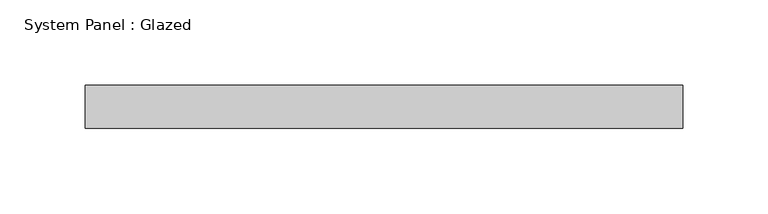
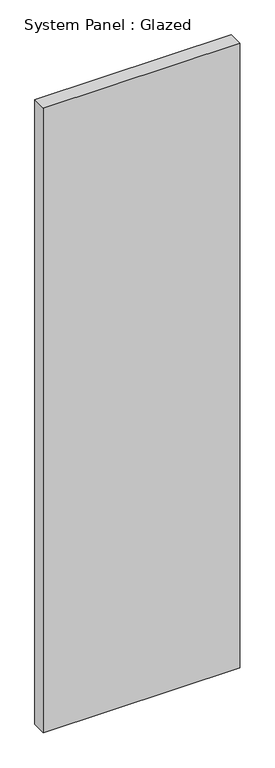
"""IFC4 building model written with IfcOpenShell, lengths in millimetres: plate geometry, System Panel : Glazed."""

from ifc_helpers import new_model, si_unit, origin, origin_with_axes, place, context, project, spatial, polyline, outline, extrude, source, transform, mapped, element, save


def system_panel_glazed_45aa6f3c(model_context):
    return source(origin(), model_context, "Body", "SweptSolid", [
        extrude(outline(polyline([(175.6833333, 19.05), (-175.6833333, 19.05), (-175.6833333, 44.45), (175.6833333, 44.45), (175.6833333, 19.05)])), origin_with_axes(), (0.0, 0.0, 1.0), 1181.1),
    ])


if __name__ == "__main__":
    model = new_model("IFC4")
    model_context = context("Model", 3, world=origin())
    ifc_project = project(units=[si_unit("LENGTHUNIT", "METRE", prefix="MILLI")], contexts=[model_context])
    site = spatial("IfcSite", under=ifc_project)
    building = spatial("IfcBuilding", under=site)
    placement = place(None, origin())
    system_panel_glazed_shape = system_panel_glazed_45aa6f3c(model_context)
    element("IfcPlate", 1, ObjectType="System Panel : Glazed", at=placement, inside=building, context=model_context, shape_type="MappedRepresentation", body=[
        mapped(system_panel_glazed_shape, transform((0.0, 0.0, 0.0), x_axis=(1.0, 0.0, 0.0), y_axis=(0.0, 1.0, 0.0), z_axis=(0.0, 0.0, 1.0))),
    ])
    save(model, "model.ifc")

# Revit data of these elements
# Type "System Panel : Glazed"
#   Construction Type Id = "GSP4R"
#   Analytic Construction = "1/8 in Pilkington single glazing"
#   Visual Light Transmittance = 0.9
#   Solar Heat Gain Coefficient = 0.86
#   Heat Transfer Coefficient (U) = 1.18115 BTU/(h·ft²·°F)
#   Define Thermal Properties by = 1
# Element 1 (IfcPlate, "System Panel : Glazed")
#   Materials on its faces: "Glass"
# Materials
#   "Glass": class "Glass", colour RGB 0 128 192, transparency 0.75, Description = "Soda Lime Glass", Cost = 0
